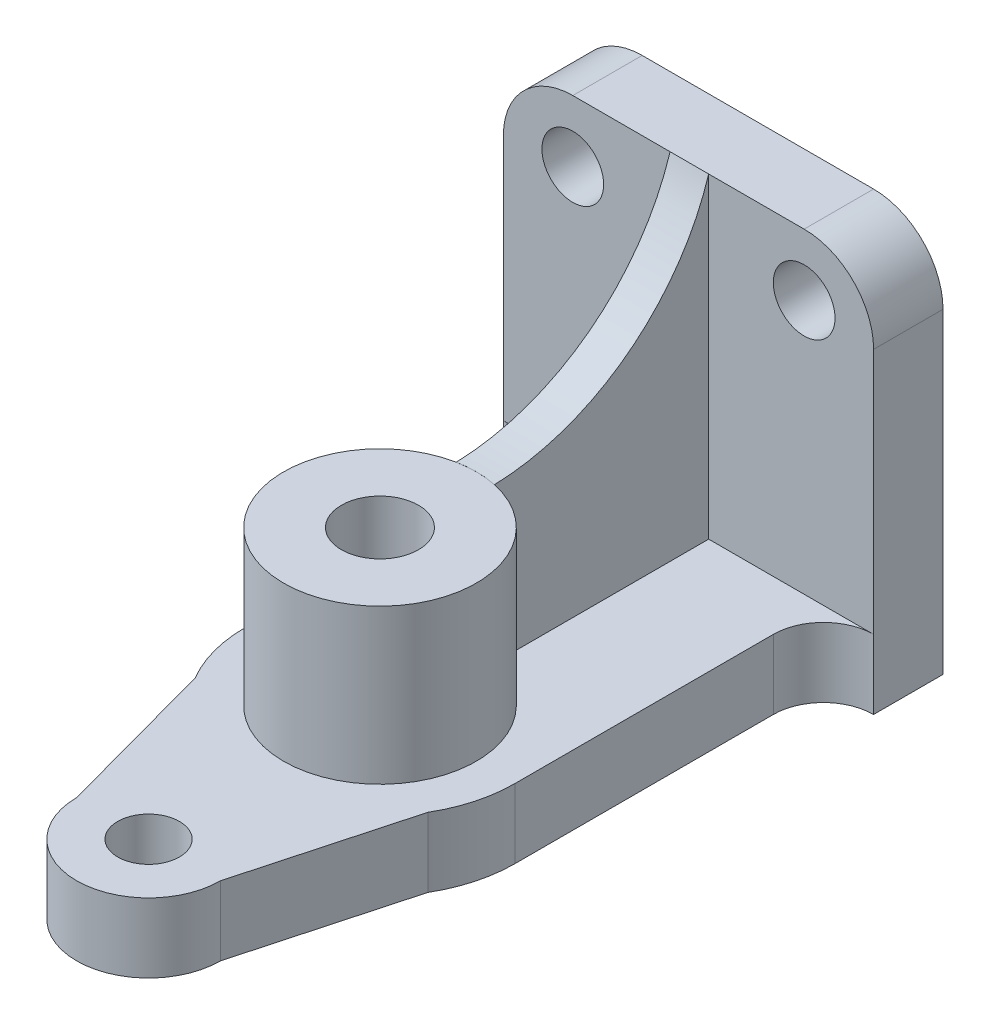
ISO-10303-21;
HEADER;
FILE_DESCRIPTION(('STEP AP214'),'2;1');
FILE_NAME('part.step','',(''),(''),'','','');
FILE_SCHEMA(('AUTOMOTIVE_DESIGN { 1 0 10303 214 1 1 1 1 }'));
ENDSEC;
DATA;
#1=APPLICATION_CONTEXT('core data for automotive mechanical design processes');
#2=APPLICATION_PROTOCOL_DEFINITION('international standard','automotive_design',2000,#1);
#3=PRODUCT_CONTEXT('',#1,'mechanical');
#4=PRODUCT('Part','Part','',(#3));
#5=PRODUCT_RELATED_PRODUCT_CATEGORY('part','',(#4));
#6=PRODUCT_DEFINITION_FORMATION('','',#4);
#7=PRODUCT_DEFINITION_CONTEXT('part definition',#1,'design');
#8=PRODUCT_DEFINITION('design','',#6,#7);
#9=PRODUCT_DEFINITION_SHAPE('','',#8);
#10=(LENGTH_UNIT() NAMED_UNIT(*) SI_UNIT(.MILLI.,.METRE.));
#11=(NAMED_UNIT(*) PLANE_ANGLE_UNIT() SI_UNIT($,.RADIAN.));
#12=(NAMED_UNIT(*) SI_UNIT($,.STERADIAN.) SOLID_ANGLE_UNIT());
#13=UNCERTAINTY_MEASURE_WITH_UNIT(LENGTH_MEASURE(1.E-05),#10,'distance_accuracy_value','');
#14=(GEOMETRIC_REPRESENTATION_CONTEXT(3) GLOBAL_UNCERTAINTY_ASSIGNED_CONTEXT((#13)) GLOBAL_UNIT_ASSIGNED_CONTEXT((#10,
#11,#12)) REPRESENTATION_CONTEXT('',''));
#15=CARTESIAN_POINT('',(0.,0.,0.));
#16=DIRECTION('',(0.,0.,1.));
#17=DIRECTION('',(1.,0.,0.));
#18=AXIS2_PLACEMENT_3D('',#15,#16,#17);
#19=CARTESIAN_POINT('',(10.,0.,78.));
#20=DIRECTION('',(-1.,0.,0.));
#21=DIRECTION('',(0.,0.,1.));
#22=AXIS2_PLACEMENT_3D('',#19,#20,#21);
#23=PLANE('',#22);
#24=CARTESIAN_POINT('',(9.99999999999999,117.976226441844,75.2438230983182));
#25=DIRECTION('',(-1.,0.,0.));
#26=DIRECTION('',(0.,0.,1.));
#27=AXIS2_PLACEMENT_3D('',#24,#25,#26);
#28=CIRCLE('',#27,60.);
#29=CARTESIAN_POINT('',(10.,58.,73.5549590432095));
#30=VERTEX_POINT('',#29);
#31=CARTESIAN_POINT('',(9.99999999999999,100.,18.));
#32=VERTEX_POINT('',#31);
#33=EDGE_CURVE('E185',#30,#32,#28,.F.);
#34=ORIENTED_EDGE('',*,*,#33,.F.);
#35=DIRECTION('',(0.,-1.,0.));
#36=VECTOR('',#35,1.);
#37=CARTESIAN_POINT('',(10.,58.,73.5549590432095));
#38=LINE('',#37,#36);
#39=CARTESIAN_POINT('',(10.,18.,73.5549590432095));
#40=VERTEX_POINT('',#39);
#41=EDGE_CURVE('E295',#30,#40,#38,.T.);
#42=ORIENTED_EDGE('',*,*,#41,.T.);
#43=DIRECTION('',(0.,0.,-1.));
#44=VECTOR('',#43,1.);
#45=CARTESIAN_POINT('',(10.,18.,78.));
#46=LINE('',#45,#44);
#47=CARTESIAN_POINT('',(10.,18.,18.));
#48=VERTEX_POINT('',#47);
#49=EDGE_CURVE('E300',#40,#48,#46,.T.);
#50=ORIENTED_EDGE('',*,*,#49,.T.);
#51=DIRECTION('',(0.,1.,0.));
#52=VECTOR('',#51,1.);
#53=CARTESIAN_POINT('',(10.,0.,18.));
#54=LINE('',#53,#52);
#55=EDGE_CURVE('E205',#48,#32,#54,.T.);
#56=ORIENTED_EDGE('',*,*,#55,.T.);
#57=EDGE_LOOP('',(#34,#42,#50,#56));
#58=FACE_BOUND('',#57,.T.);
#59=ADVANCED_FACE('F41',(#58),#23,.F.);
#60=CARTESIAN_POINT('',(0.,0.,78.));
#61=DIRECTION('',(1.,0.,0.));
#62=DIRECTION('',(0.,0.,-1.));
#63=AXIS2_PLACEMENT_3D('',#60,#61,#62);
#64=PLANE('',#63);
#65=CARTESIAN_POINT('',(0.,117.976226441844,75.2438230983182));
#66=DIRECTION('',(1.,0.,0.));
#67=DIRECTION('',(0.,0.,1.));
#68=AXIS2_PLACEMENT_3D('',#65,#66,#67);
#69=CIRCLE('',#68,60.);
#70=CARTESIAN_POINT('',(0.,58.0028187803302,73.4576614410575));
#71=VERTEX_POINT('',#70);
#72=CARTESIAN_POINT('',(0.,100.,18.));
#73=VERTEX_POINT('',#72);
#74=EDGE_CURVE('E65',#71,#73,#69,.T.);
#75=ORIENTED_EDGE('',*,*,#74,.T.);
#76=DIRECTION('',(0.,-1.,0.));
#77=VECTOR('',#76,1.);
#78=CARTESIAN_POINT('',(0.,0.,18.));
#79=LINE('',#78,#77);
#80=CARTESIAN_POINT('',(0.,18.,18.));
#81=VERTEX_POINT('',#80);
#82=EDGE_CURVE('E192',#73,#81,#79,.T.);
#83=ORIENTED_EDGE('',*,*,#82,.T.);
#84=DIRECTION('',(0.,0.,-1.));
#85=VECTOR('',#84,1.);
#86=CARTESIAN_POINT('',(0.,18.,78.));
#87=LINE('',#86,#85);
#88=CARTESIAN_POINT('',(0.,18.,73.4576614410575));
#89=VERTEX_POINT('',#88);
#90=EDGE_CURVE('E70',#89,#81,#87,.T.);
#91=ORIENTED_EDGE('',*,*,#90,.F.);
#92=DIRECTION('',(0.,-1.,0.));
#93=VECTOR('',#92,1.);
#94=CARTESIAN_POINT('',(0.,58.,73.4576614410575));
#95=LINE('',#94,#93);
#96=CARTESIAN_POINT('',(0.,58.,73.4576614410575));
#97=VERTEX_POINT('',#96);
#98=EDGE_CURVE('E292',#89,#97,#95,.F.);
#99=ORIENTED_EDGE('',*,*,#98,.T.);
#100=DIRECTION('',(0.,-1.,0.));
#101=VECTOR('',#100,1.);
#102=CARTESIAN_POINT('',(0.,138.,73.4576614410575));
#103=LINE('',#102,#101);
#104=EDGE_CURVE('E54',#71,#97,#103,.T.);
#105=ORIENTED_EDGE('',*,*,#104,.F.);
#106=EDGE_LOOP('',(#75,#83,#91,#99,#105));
#107=FACE_BOUND('',#106,.T.);
#108=ADVANCED_FACE('F195',(#107),#64,.F.);
#109=CARTESIAN_POINT('',(52.7616822718705,100.,18.));
#110=DIRECTION('',(0.,-1.,0.));
#111=DIRECTION('',(0.,0.,-1.));
#112=AXIS2_PLACEMENT_3D('',#109,#110,#111);
#113=PLANE('',#112);
#114=DIRECTION('',(-1.,0.,0.));
#115=VECTOR('',#114,1.);
#116=CARTESIAN_POINT('',(80.,100.,18.));
#117=LINE('',#116,#115);
#118=EDGE_CURVE('E177',#32,#73,#117,.T.);
#119=ORIENTED_EDGE('',*,*,#118,.F.);
#120=DIRECTION('',(-1.,0.,0.));
#121=VECTOR('',#120,1.);
#122=CARTESIAN_POINT('',(52.7616822718705,100.,18.));
#123=LINE('',#122,#121);
#124=CARTESIAN_POINT('',(34.7616822718705,100.,18.));
#125=VERTEX_POINT('',#124);
#126=EDGE_CURVE('E209',#125,#32,#123,.T.);
#127=ORIENTED_EDGE('',*,*,#126,.F.);
#128=DIRECTION('',(0.,0.,-1.));
#129=VECTOR('',#128,1.);
#130=CARTESIAN_POINT('',(34.7616822718705,100.,18.));
#131=LINE('',#130,#129);
#132=CARTESIAN_POINT('',(34.7616822718705,100.,0.));
#133=VERTEX_POINT('',#132);
#134=EDGE_CURVE('E241',#125,#133,#131,.T.);
#135=ORIENTED_EDGE('',*,*,#134,.T.);
#136=DIRECTION('',(-1.,0.,0.));
#137=VECTOR('',#136,1.);
#138=CARTESIAN_POINT('',(52.7616822718705,100.,0.));
#139=LINE('',#138,#137);
#140=CARTESIAN_POINT('',(-25.2383177281295,100.,0.));
#141=VERTEX_POINT('',#140);
#142=EDGE_CURVE('E228',#133,#141,#139,.T.);
#143=ORIENTED_EDGE('',*,*,#142,.T.);
#144=DIRECTION('',(0.,0.,-1.));
#145=VECTOR('',#144,1.);
#146=CARTESIAN_POINT('',(-25.2383177281295,100.,18.));
#147=LINE('',#146,#145);
#148=CARTESIAN_POINT('',(-25.2383177281295,100.,18.));
#149=VERTEX_POINT('',#148);
#150=EDGE_CURVE('E210',#141,#149,#147,.F.);
#151=ORIENTED_EDGE('',*,*,#150,.T.);
#152=EDGE_CURVE('E197',#73,#149,#123,.T.);
#153=ORIENTED_EDGE('',*,*,#152,.F.);
#154=EDGE_LOOP('',(#119,#127,#135,#143,#151,#153));
#155=FACE_BOUND('',#154,.T.);
#156=ADVANCED_FACE('F202',(#155),#113,.F.);
#157=CARTESIAN_POINT('',(4.76168227187048,138.,98.));
#158=DIRECTION('',(0.,-1.,0.));
#159=DIRECTION('',(1.,0.,0.));
#160=AXIS2_PLACEMENT_3D('',#157,#158,#159);
#161=CYLINDRICAL_SURFACE('',#160,25.);
#162=CARTESIAN_POINT('',(4.76168227187048,58.,98.));
#163=DIRECTION('',(0.,1.,0.));
#164=DIRECTION('',(-1.,0.,0.));
#165=AXIS2_PLACEMENT_3D('',#162,#163,#164);
#166=CIRCLE('',#165,25.);
#167=EDGE_CURVE('E283',#30,#97,#166,.T.);
#168=ORIENTED_EDGE('',*,*,#167,.F.);
#169=CARTESIAN_POINT('',(9.99999999999945,58.,73.5549590432094));
#170=CARTESIAN_POINT('',(9.65370224296303,58.0020936559718,73.4807518343738));
#171=CARTESIAN_POINT('',(9.30587160772052,58.004108949725,73.4139125284722));
#172=CARTESIAN_POINT('',(8.60767996888885,58.0078517162291,73.295066366721));
#173=CARTESIAN_POINT('',(8.25731893644608,58.0095791856927,73.2430596802795));
#174=CARTESIAN_POINT('',(7.20299529943735,58.0141342601879,73.1094028548988));
#175=CARTESIAN_POINT('',(6.49604918544244,58.0163327880321,73.0501710055342));
#176=CARTESIAN_POINT('',(5.09159762553141,58.0184740617519,72.9924584828871));
#177=CARTESIAN_POINT('',(4.39413083674992,58.0184537356825,72.9929832947581));
#178=CARTESIAN_POINT('',(3.00204216542595,58.0162552848415,73.0522866310574));
#179=CARTESIAN_POINT('',(2.30741861057202,58.0140786967999,73.1110236686719));
#180=CARTESIAN_POINT('',(1.34633053020931,58.0099258905202,73.2328901627449));
#181=CARTESIAN_POINT('',(1.07658589050279,58.0086339991649,73.2715881667999));
#182=CARTESIAN_POINT('',(0.537616896382367,58.0058566094998,73.357923069147));
#183=CARTESIAN_POINT('',(0.268397212344852,58.0043704850765,73.4055891043916));
#184=CARTESIAN_POINT('',(0.,58.0028187803302,73.4576614410575));
#185=B_SPLINE_CURVE_WITH_KNOTS('',3,(#169,#170,#171,#172,#173,#174,#175,#176,#177,#178,#179,
#180,#181,#182,#183,#184),.UNSPECIFIED.,.F.,.F.,(4,2,2,2,2,2,2,4),(0.,1.0623258838775,
2.12466390042733,4.2501259696277,6.34021977290361,8.42882507403494,9.24623962264976,
10.0663572896542),.UNSPECIFIED.);
#186=EDGE_CURVE('E11',#30,#71,#185,.T.);
#187=ORIENTED_EDGE('',*,*,#186,.T.);
#188=ORIENTED_EDGE('',*,*,#104,.T.);
#189=EDGE_LOOP('',(#168,#187,#188));
#190=FACE_BOUND('',#189,.T.);
#191=ADVANCED_FACE('F279',(#190),#161,.F.);
#192=CARTESIAN_POINT('',(0.,18.,158.));
#193=DIRECTION('',(0.,-1.,0.));
#194=DIRECTION('',(1.,0.,0.));
#195=AXIS2_PLACEMENT_3D('',#192,#193,#194);
#196=PLANE('',#195);
#197=CARTESIAN_POINT('',(4.76168227192394,18.,158.));
#198=DIRECTION('',(0.,1.,0.));
#199=DIRECTION('',(-1.,0.,0.));
#200=AXIS2_PLACEMENT_3D('',#197,#198,#199);
#201=CIRCLE('',#200,8.);
#202=CARTESIAN_POINT('',(-3.23831772807606,18.,158.));
#203=VERTEX_POINT('',#202);
#204=EDGE_CURVE('E299',#203,#203,#201,.T.);
#205=ORIENTED_EDGE('',*,*,#204,.F.);
#206=EDGE_LOOP('',(#205));
#207=FACE_BOUND('',#206,.T.);
#208=ORIENTED_EDGE('',*,*,#49,.F.);
#209=CARTESIAN_POINT('',(4.76168227187047,18.,98.));
#210=DIRECTION('',(0.,-1.,0.));
#211=DIRECTION('',(1.,0.,0.));
#212=AXIS2_PLACEMENT_3D('',#209,#210,#211);
#213=CIRCLE('',#212,25.);
#214=EDGE_CURVE('E267',#89,#40,#213,.F.);
#215=ORIENTED_EDGE('',*,*,#214,.F.);
#216=ORIENTED_EDGE('',*,*,#90,.T.);
#217=DIRECTION('',(-1.,0.,0.));
#218=VECTOR('',#217,1.);
#219=CARTESIAN_POINT('',(0.,18.,18.));
#220=LINE('',#219,#218);
#221=CARTESIAN_POINT('',(-43.2383177281295,18.,18.));
#222=VERTEX_POINT('',#221);
#223=EDGE_CURVE('E201',#81,#222,#220,.T.);
#224=ORIENTED_EDGE('',*,*,#223,.T.);
#225=CARTESIAN_POINT('',(-43.2383177281295,18.,31.));
#226=DIRECTION('',(0.,-1.,0.));
#227=DIRECTION('',(1.,0.,0.));
#228=AXIS2_PLACEMENT_3D('',#225,#226,#227);
#229=CIRCLE('',#228,13.);
#230=CARTESIAN_POINT('',(-30.2383177281295,18.,31.));
#231=VERTEX_POINT('',#230);
#232=EDGE_CURVE('E259',#222,#231,#229,.T.);
#233=ORIENTED_EDGE('',*,*,#232,.T.);
#234=DIRECTION('',(0.,0.,-1.));
#235=VECTOR('',#234,1.);
#236=CARTESIAN_POINT('',(-30.2383177281295,18.,158.));
#237=LINE('',#236,#235);
#238=CARTESIAN_POINT('',(-30.2383177281295,18.,97.9999999999999));
#239=VERTEX_POINT('',#238);
#240=EDGE_CURVE('E360',#239,#231,#237,.T.);
#241=ORIENTED_EDGE('',*,*,#240,.F.);
#242=CARTESIAN_POINT('',(4.76168227187047,18.,98.));
#243=DIRECTION('',(0.,1.,0.));
#244=DIRECTION('',(-1.,0.,0.));
#245=AXIS2_PLACEMENT_3D('',#242,#243,#244);
#246=CIRCLE('',#245,35.);
#247=CARTESIAN_POINT('',(-25.402916795203,18.,115.750970765643));
#248=VERTEX_POINT('',#247);
#249=EDGE_CURVE('E317',#239,#248,#246,.T.);
#250=ORIENTED_EDGE('',*,*,#249,.T.);
#251=DIRECTION('',(0.262825333985644,0.,0.964843429689675));
#252=VECTOR('',#251,1.);
#253=CARTESIAN_POINT('',(-53.0008998035622,18.,14.4375540774436));
#254=LINE('',#253,#252);
#255=CARTESIAN_POINT('',(-13.8941943668805,18.,158.));
#256=VERTEX_POINT('',#255);
#257=EDGE_CURVE('E316',#248,#256,#254,.T.);
#258=ORIENTED_EDGE('',*,*,#257,.T.);
#259=CARTESIAN_POINT('',(4.76168227192394,18.,158.));
#260=DIRECTION('',(0.,1.,0.));
#261=DIRECTION('',(-1.,0.,0.));
#262=AXIS2_PLACEMENT_3D('',#259,#260,#261);
#263=CIRCLE('',#262,18.6558766386789);
#264=CARTESIAN_POINT('',(23.4175589106028,18.,158.000000000068));
#265=VERTEX_POINT('',#264);
#266=EDGE_CURVE('E308',#256,#265,#263,.T.);
#267=ORIENTED_EDGE('',*,*,#266,.T.);
#268=DIRECTION('',(-0.262825333985644,0.,0.964843429689675));
#269=VECTOR('',#268,1.);
#270=CARTESIAN_POINT('',(61.8664174073116,18.,16.8525393003937));
#271=LINE('',#270,#269);
#272=CARTESIAN_POINT('',(34.9262813389439,18.,115.750970765643));
#273=VERTEX_POINT('',#272);
#274=EDGE_CURVE('E331',#273,#265,#271,.T.);
#275=ORIENTED_EDGE('',*,*,#274,.F.);
#276=CARTESIAN_POINT('',(4.76168227187047,18.,98.));
#277=DIRECTION('',(0.,1.,0.));
#278=DIRECTION('',(-1.,0.,0.));
#279=AXIS2_PLACEMENT_3D('',#276,#277,#278);
#280=CIRCLE('',#279,35.);
#281=CARTESIAN_POINT('',(39.7616822718705,18.,98.));
#282=VERTEX_POINT('',#281);
#283=EDGE_CURVE('E312',#273,#282,#280,.T.);
#284=ORIENTED_EDGE('',*,*,#283,.T.);
#285=DIRECTION('',(0.,0.,-1.));
#286=VECTOR('',#285,1.);
#287=CARTESIAN_POINT('',(39.7616822718705,18.,158.));
#288=LINE('',#287,#286);
#289=CARTESIAN_POINT('',(39.7616822718705,18.,31.));
#290=VERTEX_POINT('',#289);
#291=EDGE_CURVE('E353',#282,#290,#288,.T.);
#292=ORIENTED_EDGE('',*,*,#291,.T.);
#293=CARTESIAN_POINT('',(52.7616822718705,18.,31.));
#294=DIRECTION('',(0.,-1.,0.));
#295=DIRECTION('',(1.,0.,0.));
#296=AXIS2_PLACEMENT_3D('',#293,#294,#295);
#297=CIRCLE('',#296,13.);
#298=CARTESIAN_POINT('',(52.7616822718705,18.,18.));
#299=VERTEX_POINT('',#298);
#300=EDGE_CURVE('E266',#290,#299,#297,.T.);
#301=ORIENTED_EDGE('',*,*,#300,.T.);
#302=EDGE_CURVE('E346',#299,#48,#220,.T.);
#303=ORIENTED_EDGE('',*,*,#302,.T.);
#304=EDGE_LOOP('',(#208,#215,#216,#224,#233,#241,#250,#258,#267,#275,#284,#292,#301,#303));
#305=FACE_BOUND('',#304,.T.);
#306=ADVANCED_FACE('F396',(#207,#305),#196,.F.);
#307=CARTESIAN_POINT('',(0.,0.,18.));
#308=DIRECTION('',(0.,0.,1.));
#309=DIRECTION('',(1.,0.,0.));
#310=AXIS2_PLACEMENT_3D('',#307,#308,#309);
#311=PLANE('',#310);
#312=CARTESIAN_POINT('',(34.7616822718705,84.,18.));
#313=DIRECTION('',(0.,0.,1.));
#314=DIRECTION('',(1.,0.,0.));
#315=AXIS2_PLACEMENT_3D('',#312,#313,#314);
#316=CIRCLE('',#315,7.99999999999999);
#317=CARTESIAN_POINT('',(42.7616822718705,84.,18.));
#318=VERTEX_POINT('',#317);
#319=EDGE_CURVE('E363',#318,#318,#316,.T.);
#320=ORIENTED_EDGE('',*,*,#319,.F.);
#321=EDGE_LOOP('',(#320));
#322=FACE_BOUND('',#321,.T.);
#323=ORIENTED_EDGE('',*,*,#126,.T.);
#324=ORIENTED_EDGE('',*,*,#55,.F.);
#325=ORIENTED_EDGE('',*,*,#302,.F.);
#326=DIRECTION('',(0.,1.,0.));
#327=VECTOR('',#326,1.);
#328=CARTESIAN_POINT('',(52.7616822718705,0.,18.));
#329=LINE('',#328,#327);
#330=CARTESIAN_POINT('',(52.7616822718705,82.,18.));
#331=VERTEX_POINT('',#330);
#332=EDGE_CURVE('E213',#299,#331,#329,.T.);
#333=ORIENTED_EDGE('',*,*,#332,.T.);
#334=CARTESIAN_POINT('',(34.7616822718705,82.,18.));
#335=DIRECTION('',(0.,0.,1.));
#336=DIRECTION('',(1.,0.,0.));
#337=AXIS2_PLACEMENT_3D('',#334,#335,#336);
#338=CIRCLE('',#337,18.);
#339=EDGE_CURVE('E244',#331,#125,#338,.T.);
#340=ORIENTED_EDGE('',*,*,#339,.T.);
#341=EDGE_LOOP('',(#323,#324,#325,#333,#340));
#342=FACE_BOUND('',#341,.T.);
#343=ADVANCED_FACE('F398',(#322,#342),#311,.T.);
#344=CARTESIAN_POINT('',(-25.2383177281295,84.,18.));
#345=DIRECTION('',(0.,0.,1.));
#346=DIRECTION('',(1.,0.,0.));
#347=AXIS2_PLACEMENT_3D('',#344,#345,#346);
#348=CIRCLE('',#347,8.);
#349=CARTESIAN_POINT('',(-17.2383177281295,84.,18.));
#350=VERTEX_POINT('',#349);
#351=EDGE_CURVE('E364',#350,#350,#348,.T.);
#352=ORIENTED_EDGE('',*,*,#351,.F.);
#353=EDGE_LOOP('',(#352));
#354=FACE_BOUND('',#353,.T.);
#355=ORIENTED_EDGE('',*,*,#223,.F.);
#356=ORIENTED_EDGE('',*,*,#82,.F.);
#357=ORIENTED_EDGE('',*,*,#152,.T.);
#358=CARTESIAN_POINT('',(-25.2383177281295,82.,18.));
#359=DIRECTION('',(0.,0.,1.));
#360=DIRECTION('',(1.,0.,0.));
#361=AXIS2_PLACEMENT_3D('',#358,#359,#360);
#362=CIRCLE('',#361,18.);
#363=CARTESIAN_POINT('',(-43.2383177281295,82.,18.));
#364=VERTEX_POINT('',#363);
#365=EDGE_CURVE('E250',#149,#364,#362,.T.);
#366=ORIENTED_EDGE('',*,*,#365,.T.);
#367=DIRECTION('',(0.,-1.,0.));
#368=VECTOR('',#367,1.);
#369=CARTESIAN_POINT('',(-43.2383177281295,100.,18.));
#370=LINE('',#369,#368);
#371=EDGE_CURVE('E371',#364,#222,#370,.T.);
#372=ORIENTED_EDGE('',*,*,#371,.T.);
#373=EDGE_LOOP('',(#355,#356,#357,#366,#372));
#374=FACE_BOUND('',#373,.T.);
#375=ADVANCED_FACE('F199',(#354,#374),#311,.T.);
#376=CARTESIAN_POINT('',(4.76168227187048,58.,98.));
#377=DIRECTION('',(0.,-1.,0.));
#378=DIRECTION('',(1.,0.,0.));
#379=AXIS2_PLACEMENT_3D('',#376,#377,#378);
#380=CYLINDRICAL_SURFACE('',#379,25.);
#381=ORIENTED_EDGE('',*,*,#41,.F.);
#382=CARTESIAN_POINT('',(4.76168227187048,58.,98.));
#383=DIRECTION('',(0.,1.,0.));
#384=DIRECTION('',(-1.,0.,0.));
#385=AXIS2_PLACEMENT_3D('',#382,#383,#384);
#386=CIRCLE('',#385,25.);
#387=EDGE_CURVE('E288',#97,#30,#386,.T.);
#388=ORIENTED_EDGE('',*,*,#387,.F.);
#389=ORIENTED_EDGE('',*,*,#98,.F.);
#390=ORIENTED_EDGE('',*,*,#214,.T.);
#391=EDGE_LOOP('',(#381,#388,#389,#390));
#392=FACE_BOUND('',#391,.T.);
#393=ADVANCED_FACE('F293',(#392),#380,.T.);
#394=CARTESIAN_POINT('',(0.,58.,0.));
#395=DIRECTION('',(0.,1.,0.));
#396=DIRECTION('',(-1.,0.,0.));
#397=AXIS2_PLACEMENT_3D('',#394,#395,#396);
#398=PLANE('',#397);
#399=ORIENTED_EDGE('',*,*,#167,.T.);
#400=ORIENTED_EDGE('',*,*,#387,.T.);
#401=EDGE_LOOP('',(#399,#400));
#402=FACE_BOUND('',#401,.T.);
#403=CARTESIAN_POINT('',(4.76168227187048,58.,98.));
#404=DIRECTION('',(0.,1.,0.));
#405=DIRECTION('',(-1.,0.,0.));
#406=AXIS2_PLACEMENT_3D('',#403,#404,#405);
#407=CIRCLE('',#406,10.);
#408=CARTESIAN_POINT('',(-5.23831772812952,58.,98.));
#409=VERTEX_POINT('',#408);
#410=EDGE_CURVE('E294',#409,#409,#407,.T.);
#411=ORIENTED_EDGE('',*,*,#410,.F.);
#412=EDGE_LOOP('',(#411));
#413=FACE_BOUND('',#412,.T.);
#414=ADVANCED_FACE('F286',(#402,#413),#398,.T.);
#415=CARTESIAN_POINT('',(-43.2383177281295,0.,18.));
#416=DIRECTION('',(0.,1.,0.));
#417=DIRECTION('',(0.,0.,1.));
#418=AXIS2_PLACEMENT_3D('',#415,#416,#417);
#419=PLANE('',#418);
#420=DIRECTION('',(-0.262825333985644,0.,0.964843429689675));
#421=VECTOR('',#420,1.);
#422=CARTESIAN_POINT('',(54.3151020407067,0.,44.5737521168928));
#423=LINE('',#422,#421);
#424=CARTESIAN_POINT('',(34.9262813389439,0.,115.750970765643));
#425=VERTEX_POINT('',#424);
#426=CARTESIAN_POINT('',(23.4175589106215,0.,158.));
#427=VERTEX_POINT('',#426);
#428=EDGE_CURVE('E328',#425,#427,#423,.T.);
#429=ORIENTED_EDGE('',*,*,#428,.T.);
#430=CARTESIAN_POINT('',(4.76168227192394,0.,158.));
#431=DIRECTION('',(0.,1.,0.));
#432=DIRECTION('',(-1.,0.,0.));
#433=AXIS2_PLACEMENT_3D('',#430,#431,#432);
#434=CIRCLE('',#433,18.6558766386789);
#435=CARTESIAN_POINT('',(-13.894194366755,0.,158.));
#436=VERTEX_POINT('',#435);
#437=EDGE_CURVE('E311',#436,#427,#434,.T.);
#438=ORIENTED_EDGE('',*,*,#437,.F.);
#439=DIRECTION('',(0.262825333985644,0.,0.964843429689675));
#440=VECTOR('',#439,1.);
#441=CARTESIAN_POINT('',(-51.4231444906936,0.,20.2295636382967));
#442=LINE('',#441,#440);
#443=CARTESIAN_POINT('',(-25.402916795203,0.,115.750970765643));
#444=VERTEX_POINT('',#443);
#445=EDGE_CURVE('E339',#444,#436,#442,.T.);
#446=ORIENTED_EDGE('',*,*,#445,.F.);
#447=CARTESIAN_POINT('',(4.76168227187047,0.,98.));
#448=DIRECTION('',(0.,1.,0.));
#449=DIRECTION('',(0.,0.,1.));
#450=AXIS2_PLACEMENT_3D('',#447,#448,#449);
#451=CIRCLE('',#450,35.);
#452=CARTESIAN_POINT('',(-30.2383177281295,0.,97.9999999999999));
#453=VERTEX_POINT('',#452);
#454=EDGE_CURVE('E342',#453,#444,#451,.T.);
#455=ORIENTED_EDGE('',*,*,#454,.F.);
#456=DIRECTION('',(0.,0.,-1.));
#457=VECTOR('',#456,1.);
#458=CARTESIAN_POINT('',(-30.2383177281295,0.,158.));
#459=LINE('',#458,#457);
#460=CARTESIAN_POINT('',(-30.2383177281295,0.,31.));
#461=VERTEX_POINT('',#460);
#462=EDGE_CURVE('E357',#453,#461,#459,.T.);
#463=ORIENTED_EDGE('',*,*,#462,.T.);
#464=CARTESIAN_POINT('',(-43.2383177281295,0.,31.));
#465=DIRECTION('',(0.,1.,0.));
#466=DIRECTION('',(0.,0.,1.));
#467=AXIS2_PLACEMENT_3D('',#464,#465,#466);
#468=CIRCLE('',#467,13.);
#469=CARTESIAN_POINT('',(-43.2383177281295,0.,18.));
#470=VERTEX_POINT('',#469);
#471=EDGE_CURVE('E257',#461,#470,#468,.T.);
#472=ORIENTED_EDGE('',*,*,#471,.T.);
#473=DIRECTION('',(0.,0.,-1.));
#474=VECTOR('',#473,1.);
#475=CARTESIAN_POINT('',(-43.2383177281295,0.,18.));
#476=LINE('',#475,#474);
#477=CARTESIAN_POINT('',(-43.2383177281295,0.,0.));
#478=VERTEX_POINT('',#477);
#479=EDGE_CURVE('E233',#470,#478,#476,.T.);
#480=ORIENTED_EDGE('',*,*,#479,.T.);
#481=DIRECTION('',(1.,0.,0.));
#482=VECTOR('',#481,1.);
#483=CARTESIAN_POINT('',(-43.2383177281295,0.,0.));
#484=LINE('',#483,#482);
#485=CARTESIAN_POINT('',(52.7616822718705,0.,0.));
#486=VERTEX_POINT('',#485);
#487=EDGE_CURVE('E216',#478,#486,#484,.T.);
#488=ORIENTED_EDGE('',*,*,#487,.T.);
#489=DIRECTION('',(0.,0.,-1.));
#490=VECTOR('',#489,1.);
#491=CARTESIAN_POINT('',(52.7616822718705,0.,18.));
#492=LINE('',#491,#490);
#493=CARTESIAN_POINT('',(52.7616822718705,0.,18.));
#494=VERTEX_POINT('',#493);
#495=EDGE_CURVE('E215',#494,#486,#492,.T.);
#496=ORIENTED_EDGE('',*,*,#495,.F.);
#497=CARTESIAN_POINT('',(52.7616822718705,0.,31.));
#498=DIRECTION('',(0.,1.,0.));
#499=DIRECTION('',(0.,0.,1.));
#500=AXIS2_PLACEMENT_3D('',#497,#498,#499);
#501=CIRCLE('',#500,13.);
#502=CARTESIAN_POINT('',(39.7616822718705,0.,31.));
#503=VERTEX_POINT('',#502);
#504=EDGE_CURVE('E262',#494,#503,#501,.T.);
#505=ORIENTED_EDGE('',*,*,#504,.T.);
#506=DIRECTION('',(0.,0.,-1.));
#507=VECTOR('',#506,1.);
#508=CARTESIAN_POINT('',(39.7616822718705,0.,158.));
#509=LINE('',#508,#507);
#510=CARTESIAN_POINT('',(39.7616822718705,0.,98.));
#511=VERTEX_POINT('',#510);
#512=EDGE_CURVE('E354',#511,#503,#509,.T.);
#513=ORIENTED_EDGE('',*,*,#512,.F.);
#514=CARTESIAN_POINT('',(4.76168227187047,0.,98.));
#515=DIRECTION('',(0.,1.,0.));
#516=DIRECTION('',(0.,0.,1.));
#517=AXIS2_PLACEMENT_3D('',#514,#515,#516);
#518=CIRCLE('',#517,35.);
#519=EDGE_CURVE('E341',#425,#511,#518,.T.);
#520=ORIENTED_EDGE('',*,*,#519,.F.);
#521=EDGE_LOOP('',(#429,#438,#446,#455,#463,#472,#480,#488,#496,#505,#513,#520));
#522=FACE_BOUND('',#521,.T.);
#523=CARTESIAN_POINT('',(4.76168227192394,0.,158.));
#524=DIRECTION('',(0.,1.,0.));
#525=DIRECTION('',(-1.,0.,0.));
#526=AXIS2_PLACEMENT_3D('',#523,#524,#525);
#527=CIRCLE('',#526,8.);
#528=CARTESIAN_POINT('',(-3.23831772807606,0.,158.));
#529=VERTEX_POINT('',#528);
#530=EDGE_CURVE('E304',#529,#529,#527,.T.);
#531=ORIENTED_EDGE('',*,*,#530,.T.);
#532=EDGE_LOOP('',(#531));
#533=FACE_BOUND('',#532,.T.);
#534=ADVANCED_FACE('F390',(#522,#533),#419,.F.);
#535=CARTESIAN_POINT('',(-43.2383177281295,100.,18.));
#536=DIRECTION('',(1.,0.,0.));
#537=DIRECTION('',(0.,0.,-1.));
#538=AXIS2_PLACEMENT_3D('',#535,#536,#537);
#539=PLANE('',#538);
#540=ORIENTED_EDGE('',*,*,#371,.F.);
#541=DIRECTION('',(0.,0.,-1.));
#542=VECTOR('',#541,1.);
#543=CARTESIAN_POINT('',(-43.2383177281295,82.,18.));
#544=LINE('',#543,#542);
#545=CARTESIAN_POINT('',(-43.2383177281295,82.,0.));
#546=VERTEX_POINT('',#545);
#547=EDGE_CURVE('E234',#364,#546,#544,.T.);
#548=ORIENTED_EDGE('',*,*,#547,.T.);
#549=DIRECTION('',(0.,-1.,0.));
#550=VECTOR('',#549,1.);
#551=CARTESIAN_POINT('',(-43.2383177281295,100.,0.));
#552=LINE('',#551,#550);
#553=EDGE_CURVE('E217',#546,#478,#552,.T.);
#554=ORIENTED_EDGE('',*,*,#553,.T.);
#555=ORIENTED_EDGE('',*,*,#479,.F.);
#556=EDGE_CURVE('E226',#222,#470,#370,.T.);
#557=ORIENTED_EDGE('',*,*,#556,.F.);
#558=EDGE_LOOP('',(#540,#548,#554,#555,#557));
#559=FACE_BOUND('',#558,.T.);
#560=ADVANCED_FACE('F385',(#559),#539,.F.);
#561=CARTESIAN_POINT('',(52.7616822718705,0.,18.));
#562=DIRECTION('',(-1.,0.,0.));
#563=DIRECTION('',(0.,0.,1.));
#564=AXIS2_PLACEMENT_3D('',#561,#562,#563);
#565=PLANE('',#564);
#566=DIRECTION('',(0.,1.,0.));
#567=VECTOR('',#566,1.);
#568=CARTESIAN_POINT('',(52.7616822718705,0.,0.));
#569=LINE('',#568,#567);
#570=CARTESIAN_POINT('',(52.7616822718705,82.,0.));
#571=VERTEX_POINT('',#570);
#572=EDGE_CURVE('E223',#486,#571,#569,.T.);
#573=ORIENTED_EDGE('',*,*,#572,.T.);
#574=DIRECTION('',(0.,0.,-1.));
#575=VECTOR('',#574,1.);
#576=CARTESIAN_POINT('',(52.7616822718705,82.,18.));
#577=LINE('',#576,#575);
#578=EDGE_CURVE('E248',#571,#331,#577,.F.);
#579=ORIENTED_EDGE('',*,*,#578,.T.);
#580=ORIENTED_EDGE('',*,*,#332,.F.);
#581=EDGE_CURVE('E208',#494,#299,#329,.T.);
#582=ORIENTED_EDGE('',*,*,#581,.F.);
#583=ORIENTED_EDGE('',*,*,#495,.T.);
#584=EDGE_LOOP('',(#573,#579,#580,#582,#583));
#585=FACE_BOUND('',#584,.T.);
#586=ADVANCED_FACE('F487',(#585),#565,.F.);
#587=CARTESIAN_POINT('',(0.,0.,0.));
#588=DIRECTION('',(0.,0.,1.));
#589=DIRECTION('',(1.,0.,0.));
#590=AXIS2_PLACEMENT_3D('',#587,#588,#589);
#591=PLANE('',#590);
#592=CARTESIAN_POINT('',(-25.2383177281295,84.,0.));
#593=DIRECTION('',(0.,0.,1.));
#594=DIRECTION('',(1.,0.,0.));
#595=AXIS2_PLACEMENT_3D('',#592,#593,#594);
#596=CIRCLE('',#595,8.);
#597=CARTESIAN_POINT('',(-17.2383177281295,84.,0.));
#598=VERTEX_POINT('',#597);
#599=EDGE_CURVE('E221',#598,#598,#596,.T.);
#600=ORIENTED_EDGE('',*,*,#599,.T.);
#601=EDGE_LOOP('',(#600));
#602=FACE_BOUND('',#601,.T.);
#603=CARTESIAN_POINT('',(34.7616822718705,84.,0.));
#604=DIRECTION('',(0.,0.,1.));
#605=DIRECTION('',(1.,0.,0.));
#606=AXIS2_PLACEMENT_3D('',#603,#604,#605);
#607=CIRCLE('',#606,7.99999999999999);
#608=CARTESIAN_POINT('',(42.7616822718705,84.,0.));
#609=VERTEX_POINT('',#608);
#610=EDGE_CURVE('E370',#609,#609,#607,.T.);
#611=ORIENTED_EDGE('',*,*,#610,.T.);
#612=EDGE_LOOP('',(#611));
#613=FACE_BOUND('',#612,.T.);
#614=ORIENTED_EDGE('',*,*,#553,.F.);
#615=CARTESIAN_POINT('',(-25.2383177281295,82.,0.));
#616=DIRECTION('',(0.,0.,1.));
#617=DIRECTION('',(1.,0.,0.));
#618=AXIS2_PLACEMENT_3D('',#615,#616,#617);
#619=CIRCLE('',#618,18.);
#620=EDGE_CURVE('E237',#546,#141,#619,.F.);
#621=ORIENTED_EDGE('',*,*,#620,.T.);
#622=ORIENTED_EDGE('',*,*,#142,.F.);
#623=CARTESIAN_POINT('',(34.7616822718705,82.,0.));
#624=DIRECTION('',(0.,0.,1.));
#625=DIRECTION('',(1.,0.,0.));
#626=AXIS2_PLACEMENT_3D('',#623,#624,#625);
#627=CIRCLE('',#626,18.);
#628=EDGE_CURVE('E240',#133,#571,#627,.F.);
#629=ORIENTED_EDGE('',*,*,#628,.T.);
#630=ORIENTED_EDGE('',*,*,#572,.F.);
#631=ORIENTED_EDGE('',*,*,#487,.F.);
#632=EDGE_LOOP('',(#614,#621,#622,#629,#630,#631));
#633=FACE_BOUND('',#632,.T.);
#634=ADVANCED_FACE('F500',(#602,#613,#633),#591,.F.);
#635=CARTESIAN_POINT('',(34.7616822718705,84.,0.));
#636=DIRECTION('',(0.,0.,1.));
#637=DIRECTION('',(1.,0.,0.));
#638=AXIS2_PLACEMENT_3D('',#635,#636,#637);
#639=CYLINDRICAL_SURFACE('',#638,7.99999999999999);
#640=ORIENTED_EDGE('',*,*,#610,.F.);
#641=EDGE_LOOP('',(#640));
#642=FACE_BOUND('',#641,.T.);
#643=ORIENTED_EDGE('',*,*,#319,.T.);
#644=EDGE_LOOP('',(#643));
#645=FACE_BOUND('',#644,.T.);
#646=ADVANCED_FACE('F508',(#642,#645),#639,.F.);
#647=CARTESIAN_POINT('',(-25.2383177281295,84.,0.));
#648=DIRECTION('',(0.,0.,1.));
#649=DIRECTION('',(1.,0.,0.));
#650=AXIS2_PLACEMENT_3D('',#647,#648,#649);
#651=CYLINDRICAL_SURFACE('',#650,8.);
#652=ORIENTED_EDGE('',*,*,#599,.F.);
#653=EDGE_LOOP('',(#652));
#654=FACE_BOUND('',#653,.T.);
#655=ORIENTED_EDGE('',*,*,#351,.T.);
#656=EDGE_LOOP('',(#655));
#657=FACE_BOUND('',#656,.T.);
#658=ADVANCED_FACE('F466',(#654,#657),#651,.F.);
#659=CARTESIAN_POINT('',(-25.2383177281295,82.,18.));
#660=DIRECTION('',(0.,0.,-1.));
#661=DIRECTION('',(-1.,0.,0.));
#662=AXIS2_PLACEMENT_3D('',#659,#660,#661);
#663=CYLINDRICAL_SURFACE('',#662,18.);
#664=ORIENTED_EDGE('',*,*,#365,.F.);
#665=ORIENTED_EDGE('',*,*,#150,.F.);
#666=ORIENTED_EDGE('',*,*,#620,.F.);
#667=ORIENTED_EDGE('',*,*,#547,.F.);
#668=EDGE_LOOP('',(#664,#665,#666,#667));
#669=FACE_BOUND('',#668,.T.);
#670=ADVANCED_FACE('F461',(#669),#663,.T.);
#671=CARTESIAN_POINT('',(34.7616822718705,82.,18.));
#672=DIRECTION('',(0.,0.,-1.));
#673=DIRECTION('',(-1.,0.,0.));
#674=AXIS2_PLACEMENT_3D('',#671,#672,#673);
#675=CYLINDRICAL_SURFACE('',#674,18.);
#676=ORIENTED_EDGE('',*,*,#339,.F.);
#677=ORIENTED_EDGE('',*,*,#578,.F.);
#678=ORIENTED_EDGE('',*,*,#628,.F.);
#679=ORIENTED_EDGE('',*,*,#134,.F.);
#680=EDGE_LOOP('',(#676,#677,#678,#679));
#681=FACE_BOUND('',#680,.T.);
#682=ADVANCED_FACE('F459',(#681),#675,.T.);
#683=CARTESIAN_POINT('',(-30.2383177281295,0.,158.));
#684=DIRECTION('',(1.,0.,0.));
#685=DIRECTION('',(0.,0.,-1.));
#686=AXIS2_PLACEMENT_3D('',#683,#684,#685);
#687=PLANE('',#686);
#688=ORIENTED_EDGE('',*,*,#462,.F.);
#689=DIRECTION('',(0.,1.,0.));
#690=VECTOR('',#689,1.);
#691=CARTESIAN_POINT('',(-30.2383177281295,-22.,97.9999999999999));
#692=LINE('',#691,#690);
#693=EDGE_CURVE('E322',#453,#239,#692,.T.);
#694=ORIENTED_EDGE('',*,*,#693,.T.);
#695=ORIENTED_EDGE('',*,*,#240,.T.);
#696=DIRECTION('',(0.,-1.,0.));
#697=VECTOR('',#696,1.);
#698=CARTESIAN_POINT('',(-30.2383177281295,0.,31.));
#699=LINE('',#698,#697);
#700=EDGE_CURVE('E255',#231,#461,#699,.T.);
#701=ORIENTED_EDGE('',*,*,#700,.T.);
#702=EDGE_LOOP('',(#688,#694,#695,#701));
#703=FACE_BOUND('',#702,.T.);
#704=ADVANCED_FACE('F395',(#703),#687,.F.);
#705=CARTESIAN_POINT('',(39.7616822718705,0.,158.));
#706=DIRECTION('',(1.,0.,0.));
#707=DIRECTION('',(0.,0.,-1.));
#708=AXIS2_PLACEMENT_3D('',#705,#706,#707);
#709=PLANE('',#708);
#710=DIRECTION('',(0.,1.,0.));
#711=VECTOR('',#710,1.);
#712=CARTESIAN_POINT('',(39.7616822718705,-22.,98.));
#713=LINE('',#712,#711);
#714=EDGE_CURVE('E318',#511,#282,#713,.T.);
#715=ORIENTED_EDGE('',*,*,#714,.F.);
#716=ORIENTED_EDGE('',*,*,#512,.T.);
#717=DIRECTION('',(0.,-1.,0.));
#718=VECTOR('',#717,1.);
#719=CARTESIAN_POINT('',(39.7616822718705,18.,31.));
#720=LINE('',#719,#718);
#721=EDGE_CURVE('E253',#503,#290,#720,.F.);
#722=ORIENTED_EDGE('',*,*,#721,.T.);
#723=ORIENTED_EDGE('',*,*,#291,.F.);
#724=EDGE_LOOP('',(#715,#716,#722,#723));
#725=FACE_BOUND('',#724,.T.);
#726=ADVANCED_FACE('F452',(#725),#709,.T.);
#727=CARTESIAN_POINT('',(-43.2383177281295,0.,31.));
#728=DIRECTION('',(0.,-1.,0.));
#729=DIRECTION('',(0.,0.,-1.));
#730=AXIS2_PLACEMENT_3D('',#727,#728,#729);
#731=CYLINDRICAL_SURFACE('',#730,13.);
#732=ORIENTED_EDGE('',*,*,#232,.F.);
#733=ORIENTED_EDGE('',*,*,#556,.T.);
#734=ORIENTED_EDGE('',*,*,#471,.F.);
#735=ORIENTED_EDGE('',*,*,#700,.F.);
#736=EDGE_LOOP('',(#732,#733,#734,#735));
#737=FACE_BOUND('',#736,.T.);
#738=ADVANCED_FACE('F377',(#737),#731,.F.);
#739=CARTESIAN_POINT('',(52.7616822718705,0.,31.));
#740=DIRECTION('',(0.,1.,0.));
#741=DIRECTION('',(0.,0.,1.));
#742=AXIS2_PLACEMENT_3D('',#739,#740,#741);
#743=CYLINDRICAL_SURFACE('',#742,13.);
#744=ORIENTED_EDGE('',*,*,#300,.F.);
#745=ORIENTED_EDGE('',*,*,#721,.F.);
#746=ORIENTED_EDGE('',*,*,#504,.F.);
#747=ORIENTED_EDGE('',*,*,#581,.T.);
#748=EDGE_LOOP('',(#744,#745,#746,#747));
#749=FACE_BOUND('',#748,.T.);
#750=ADVANCED_FACE('F43',(#749),#743,.F.);
#751=CARTESIAN_POINT('',(4.76168227187048,58.,98.));
#752=DIRECTION('',(0.,-1.,0.));
#753=DIRECTION('',(1.,0.,0.));
#754=AXIS2_PLACEMENT_3D('',#751,#752,#753);
#755=CYLINDRICAL_SURFACE('',#754,10.);
#756=ORIENTED_EDGE('',*,*,#410,.T.);
#757=EDGE_LOOP('',(#756));
#758=FACE_BOUND('',#757,.T.);
#759=CARTESIAN_POINT('',(4.76168227187047,18.,98.));
#760=DIRECTION('',(0.,1.,0.));
#761=DIRECTION('',(-1.,0.,0.));
#762=AXIS2_PLACEMENT_3D('',#759,#760,#761);
#763=CIRCLE('',#762,10.);
#764=CARTESIAN_POINT('',(-5.23831772812953,18.,98.));
#765=VERTEX_POINT('',#764);
#766=EDGE_CURVE('E344',#765,#765,#763,.T.);
#767=ORIENTED_EDGE('',*,*,#766,.F.);
#768=EDGE_LOOP('',(#767));
#769=FACE_BOUND('',#768,.T.);
#770=ADVANCED_FACE('F411',(#758,#769),#755,.F.);
#771=ORIENTED_EDGE('',*,*,#766,.T.);
#772=EDGE_LOOP('',(#771));
#773=FACE_BOUND('',#772,.T.);
#774=ADVANCED_FACE('F402',(#773),#196,.F.);
#775=CARTESIAN_POINT('',(4.76168227187047,-22.,98.));
#776=DIRECTION('',(0.,1.,0.));
#777=DIRECTION('',(-1.,0.,0.));
#778=AXIS2_PLACEMENT_3D('',#775,#776,#777);
#779=CYLINDRICAL_SURFACE('',#778,35.);
#780=ORIENTED_EDGE('',*,*,#519,.T.);
#781=ORIENTED_EDGE('',*,*,#714,.T.);
#782=ORIENTED_EDGE('',*,*,#283,.F.);
#783=DIRECTION('',(0.,1.,0.));
#784=VECTOR('',#783,1.);
#785=CARTESIAN_POINT('',(34.9262813389439,-22.,115.750970765643));
#786=LINE('',#785,#784);
#787=EDGE_CURVE('E332',#425,#273,#786,.T.);
#788=ORIENTED_EDGE('',*,*,#787,.F.);
#789=EDGE_LOOP('',(#780,#781,#782,#788));
#790=FACE_BOUND('',#789,.T.);
#791=ADVANCED_FACE('F415',(#790),#779,.T.);
#792=CARTESIAN_POINT('',(61.8664174073116,-22.,16.8525393003937));
#793=DIRECTION('',(-0.964843429689675,0.,-0.262825333985644));
#794=DIRECTION('',(-0.262825333985644,0.,0.964843429689675));
#795=AXIS2_PLACEMENT_3D('',#792,#793,#794);
#796=PLANE('',#795);
#797=ORIENTED_EDGE('',*,*,#787,.T.);
#798=ORIENTED_EDGE('',*,*,#274,.T.);
#799=DIRECTION('',(0.,-1.,0.));
#800=VECTOR('',#799,1.);
#801=CARTESIAN_POINT('',(23.4175589106215,0.,158.));
#802=LINE('',#801,#800);
#803=EDGE_CURVE('E275',#265,#427,#802,.T.);
#804=ORIENTED_EDGE('',*,*,#803,.T.);
#805=ORIENTED_EDGE('',*,*,#428,.F.);
#806=EDGE_LOOP('',(#797,#798,#804,#805));
#807=FACE_BOUND('',#806,.T.);
#808=ADVANCED_FACE('F438',(#807),#796,.F.);
#809=CARTESIAN_POINT('',(4.76168227187047,-22.,98.));
#810=DIRECTION('',(0.,1.,0.));
#811=DIRECTION('',(-1.,0.,0.));
#812=AXIS2_PLACEMENT_3D('',#809,#810,#811);
#813=CYLINDRICAL_SURFACE('',#812,35.);
#814=ORIENTED_EDGE('',*,*,#454,.T.);
#815=DIRECTION('',(0.,1.,0.));
#816=VECTOR('',#815,1.);
#817=CARTESIAN_POINT('',(-25.402916795203,-22.,115.750970765643));
#818=LINE('',#817,#816);
#819=EDGE_CURVE('E323',#444,#248,#818,.T.);
#820=ORIENTED_EDGE('',*,*,#819,.T.);
#821=ORIENTED_EDGE('',*,*,#249,.F.);
#822=ORIENTED_EDGE('',*,*,#693,.F.);
#823=EDGE_LOOP('',(#814,#820,#821,#822));
#824=FACE_BOUND('',#823,.T.);
#825=ADVANCED_FACE('F432',(#824),#813,.T.);
#826=CARTESIAN_POINT('',(-53.0008998035622,-22.,14.4375540774436));
#827=DIRECTION('',(-0.964843429689675,0.,0.262825333985644));
#828=DIRECTION('',(0.262825333985644,0.,0.964843429689675));
#829=AXIS2_PLACEMENT_3D('',#826,#827,#828);
#830=PLANE('',#829);
#831=ORIENTED_EDGE('',*,*,#445,.T.);
#832=DIRECTION('',(0.,-1.,0.));
#833=VECTOR('',#832,1.);
#834=CARTESIAN_POINT('',(-13.8941943668805,0.,158.));
#835=LINE('',#834,#833);
#836=EDGE_CURVE('E273',#256,#436,#835,.T.);
#837=ORIENTED_EDGE('',*,*,#836,.F.);
#838=ORIENTED_EDGE('',*,*,#257,.F.);
#839=ORIENTED_EDGE('',*,*,#819,.F.);
#840=EDGE_LOOP('',(#831,#837,#838,#839));
#841=FACE_BOUND('',#840,.T.);
#842=ADVANCED_FACE('F427',(#841),#830,.T.);
#843=CARTESIAN_POINT('',(4.76168227192394,0.,158.));
#844=DIRECTION('',(0.,1.,0.));
#845=DIRECTION('',(-1.,0.,0.));
#846=AXIS2_PLACEMENT_3D('',#843,#844,#845);
#847=CYLINDRICAL_SURFACE('',#846,18.6558766386789);
#848=ORIENTED_EDGE('',*,*,#803,.F.);
#849=ORIENTED_EDGE('',*,*,#266,.F.);
#850=ORIENTED_EDGE('',*,*,#836,.T.);
#851=ORIENTED_EDGE('',*,*,#437,.T.);
#852=EDGE_LOOP('',(#848,#849,#850,#851));
#853=FACE_BOUND('',#852,.T.);
#854=ADVANCED_FACE('F428',(#853),#847,.T.);
#855=CARTESIAN_POINT('',(4.76168227192394,0.,158.));
#856=DIRECTION('',(0.,1.,0.));
#857=DIRECTION('',(-1.,0.,0.));
#858=AXIS2_PLACEMENT_3D('',#855,#856,#857);
#859=CYLINDRICAL_SURFACE('',#858,8.);
#860=ORIENTED_EDGE('',*,*,#204,.T.);
#861=EDGE_LOOP('',(#860));
#862=FACE_BOUND('',#861,.T.);
#863=ORIENTED_EDGE('',*,*,#530,.F.);
#864=EDGE_LOOP('',(#863));
#865=FACE_BOUND('',#864,.T.);
#866=ADVANCED_FACE('F425',(#862,#865),#859,.F.);
#867=CARTESIAN_POINT('',(80.,117.976226441844,75.2438230983182));
#868=DIRECTION('',(-1.,0.,0.));
#869=DIRECTION('',(0.,0.,1.));
#870=AXIS2_PLACEMENT_3D('',#867,#868,#869);
#871=CYLINDRICAL_SURFACE('',#870,60.);
#872=ORIENTED_EDGE('',*,*,#33,.T.);
#873=ORIENTED_EDGE('',*,*,#118,.T.);
#874=ORIENTED_EDGE('',*,*,#74,.F.);
#875=ORIENTED_EDGE('',*,*,#186,.F.);
#876=EDGE_LOOP('',(#872,#873,#874,#875));
#877=FACE_BOUND('',#876,.T.);
#878=ADVANCED_FACE('F179',(#877),#871,.F.);
#879=CLOSED_SHELL('',(#59,#108,#156,#191,#306,#343,#375,#393,#414,#534,#560,#586,#634,#646,#658,
#670,#682,#704,#726,#738,#750,#770,#774,#791,#808,#825,#842,#854,#866,#878));
#880=MANIFOLD_SOLID_BREP('B2',#879);
#881=ADVANCED_BREP_SHAPE_REPRESENTATION('',(#18,#880),#14);
#882=SHAPE_DEFINITION_REPRESENTATION(#9,#881);
ENDSEC;
END-ISO-10303-21;
